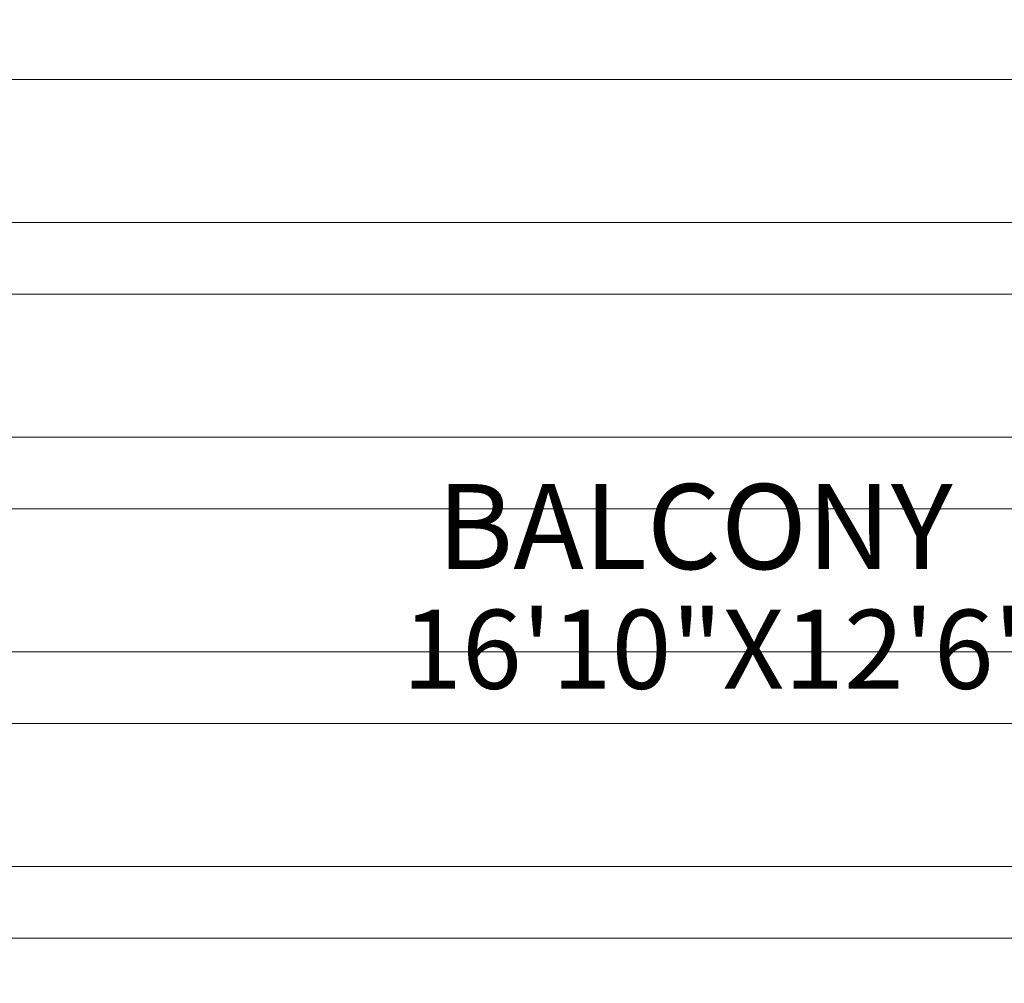
# Model space of a CAD drawing. Units: inches. Extents: x 351 to 1738, y -265 to 286.
# Tile 14 of 38: x 1090 to 1176, y -147 to -63. Entities that reach past the tile are written whole.
import ezdxf

# ---------------------------------------------------------------- set-up
doc = ezdxf.new("R2010")
doc.units = ezdxf.units.IN
doc.header["$MEASUREMENT"] = 0
doc.layers.add('A-AREA-IDEN', color=7, linetype='Continuous', lineweight=18)
doc.layers.add('A-FLOR-PATT', color=9, linetype='Continuous', lineweight=9)
doc.styles.add('Annotative', font='arial.ttf')

msp = doc.modelspace()

# ---------------------------------------------------------------- hatches: boundary and pattern name
at = {"layer": 'A-FLOR-PATT', "transparency": 33554559}
h = msp.add_hatch(dxfattribs=at)
h.set_pattern_fill('ANSI37', color=256, scale=200, angle=135)
h.set_pattern_definition([(180, (1112.704, -164.037), (-2e-15, -25), []), (270, (1112.704, -164.037), (25, -5e-15), [])])
h.paths.add_polyline_path([(1380.064, 73.463), (1380.132, 148.463), (1338.064, 148.463), (1290.704, 148.463), (1290.704, 88.463), (1248.704, 88.463), (1248.704, -2.009), (1244.704, -2.009), (1244.704, 142.457), (1160.704, 142.457), (1160.704, 158.963), (1160.704, 170.137), (1160.704, 206.137), (1160.704, 228.963), (1112.704, 228.963), (1112.704, 209.963), (1112.704, 168.963), (1124.704, 168.963), (1124.704, 162.963), (1112.704, 162.963), (1112.704, 64.463), (1112.704, 60.463), (1112.704, 0.463), (1112.704, -48.026), (1146.804, -47.981), (1146.804, -35.691), (1207.804, -35.691), (1207.804, -47.902), (1236.542, -47.864), (1236.544, -50.009), (1248.5, -50.009), (1248.506, -102.915), (1248.512, -150.915), (1248.514, -164.037), (1248.549, -164.037), (1273.017, -164.037), (1273.017, -128.799), (1355.24, -128.799), (1355.24, -164.037), (1384.204, -164.037), (1384.204, -57.037), (1380.064, -57.037), (1380.064, -48.037), (1392.064, -48.037), (1392.064, -53.037), (1406.549, -53.037), (1406.549, -57.037), (1401.204, -57.037), (1401.204, -147.037), (1468.204, -147.037), (1468.204, -138.5), (1472.204, -138.5), (1472.204, -102.5), (1468.204, -102.5), (1468.204, -57.037), (1442.549, -57.037), (1442.549, -53.037), (1463.049, -53.037), (1463.049, -40.747), (1524.049, -40.747), (1524.049, -48.037), (1536.064, -48.037), (1536.064, -53.037), (1557.704, -53.037), (1557.704, 204.963), (1384.204, 204.963), (1384.204, 73.463), (1392.064, 73.463), (1392.064, 64.463), (1384.204, 64.463), (1384.204, -3.5), (1380.204, -3.537), (1380.204, 64.463), (1380.064, 64.463)])
h.paths.add_polyline_path([(1510.714, 86.458, -0.103984), (1511.661, 85.595, 0.470438), (1510.158, 87.614, 0.0961)], flags=16)
h.paths.add_polyline_path([(1510.443, 100.266, 0.009798), (1504.693, 100.48, 0.02879), (1504.6, 99.767, -0.165331), (1505.519, 96.135, -0.143601)], flags=16)
h.paths.add_polyline_path([(1487.201, 85.595, -0.103984), (1488.148, 86.458, 0.0961), (1488.704, 87.614, 0.470438)], flags=0)
h.paths.add_polyline_path([(1495.052, 100.43), (1494.178, 100.43, -0.026463), (1494.262, 99.774, -0.144219)], flags=16)
h.paths.add_polyline_path([(1444.485, 86.458, -0.103984), (1445.433, 85.595, 0.470438), (1443.93, 87.614, 0.0961)], flags=16)
h.paths.add_polyline_path([(1420.972, 85.595, -0.103984), (1421.92, 86.458, 0.0961), (1422.475, 87.614, 0.470438)], flags=16)
h.paths.add_polyline_path([(1428.632, 100.335, 0.001054), (1427.971, 100.309, -0.021524), (1428.033, 99.774, -0.114301)], flags=16)
h.paths.add_polyline_path([(1419.906, 143.708, 0.024979), (1420.222, 157.526), (1421.573, 159.101), (1421.573, 175.369), (1391.393, 175.369), (1391.393, 200.519), (1542.294, 200.519), (1542.294, 175.369), (1512.028, 175.369, 0.019865), (1511.521, 153.838, 0.025134), (1512.758, 118.323, 0.020553), (1512.942, 115.253), (1419.834, 115.253, -0.000414), (1419.843, 124.798), (1413.059, 124.798), (1413.059, 84.437, -0.061853), (1415.831, 80.45, -0.093077), (1420.972, 85.595, -0.267537), (1422.371, 84.732, 0.08511), (1424.052, 84.616, -0.885393), (1424.033, 84.851, -1.125815), (1424.073, 84.366, -0.087987), (1422.371, 84.732, -0.267537), (1422.326, 83.089, -0.370542), (1420.972, 85.595, 0.093077), (1415.831, 80.45, -0.087414), (1417.914, 73.937), (1418.941, 73.937, 0.02725), (1418.913, 76.906, -0.115703), (1421.051, 73.937), (1445.354, 73.937, -0.115703), (1447.492, 76.906, 0.02725), (1447.464, 73.937), (1448.491, 73.937, -0.087414), (1450.574, 80.45, 0.093077), (1445.433, 85.595, -0.370542), (1444.079, 83.089, -0.267537), (1444.034, 84.732, -0.087987), (1442.332, 84.366, -1.125815), (1442.372, 84.851, -2.032736), (1442.364, 84.368, 0.086378), (1444.034, 84.732, -0.267537), (1445.433, 85.595, -0.093077), (1450.574, 80.45, -0.257732), (1466.483, 90.927, -0.47867), (1468.832, 91.907, -0.47867), (1471.18, 90.927, -0.26264), (1483.053, 81.78, -0.071866), (1487.201, 85.595, -0.267537), (1488.6, 84.732, 0.08511), (1490.28, 84.616, -0.885393), (1490.262, 84.851, -1.125815), (1490.301, 84.366, -0.087987), (1488.6, 84.732, -0.267537), (1488.554, 83.089, -0.370542), (1487.201, 85.595, 0.071866), (1483.053, 81.78, -0.132065), (1484.143, 73.937), (1485.169, 73.937, 0.02725), (1485.142, 76.906, -0.115703), (1487.28, 73.937), (1511.582, 73.937, -0.115703), (1513.72, 76.906, 0.02725), (1513.693, 73.937), (1514.719, 73.937, -0.087414), (1516.802, 80.45, 0.093077), (1511.661, 85.595, -0.370542), (1510.308, 83.089, -0.267537), (1510.262, 84.732, -0.087987), (1508.561, 84.366, -1.125815), (1508.601, 84.851, -2.032736), (1508.592, 84.368, 0.086378), (1510.262, 84.732, -0.267537), (1511.661, 85.595, -0.093077), (1516.802, 80.45, -0.061853), (1519.575, 84.437), (1519.575, 73.937), (1413.059, 73.937), (1413.059, 124.798), (1419.843, 124.798, -0.000821)], flags=16)
h.paths.add_polyline_path([(1220.149, 54.133, -0.103984), (1220.869, 53.476, 0.470438), (1219.727, 55.011, 0.0961)], flags=16)
h.paths.add_polyline_path([(1219.944, 64.626, 0.009798), (1215.574, 64.789, 0.02879), (1215.503, 64.247, -0.165331), (1216.201, 61.487, -0.143601)], flags=16)
h.paths.add_polyline_path([(1209.779, 64.449, 0.097446), (1209.339, 64.751), (1208.247, 64.751, 0.12739), (1207.7, 64.326, 0.171586), (1206.95, 61.475, -0.158854), (1207.636, 59.45, 0.015898), (1207.795, 59.218, 0.061546), (1208.598, 59.616, 0.175416), (1208.638, 60.099, -0.284779), (1209.348, 62.472, 0.326216)], flags=16)
h.paths.add_polyline_path([(1169.818, 54.133, -0.103984), (1170.538, 53.476, 0.470438), (1169.396, 55.011, 0.0961)], flags=16)
h.paths.add_polyline_path([(1159.017, 62.472, 0.284764), (1158.307, 60.099, -0.175433), (1158.267, 59.616, 0.39293), (1159.448, 64.449, -0.32623)], flags=16)
h.paths.add_polyline_path([(1156.342, 58.239, -0.178321), (1154.011, 55.31, -0.174736), (1154.722, 55.233, -0.200802), (1156.27, 56.086, 0.12699), (1157.283, 58.991, -0.091205)], flags=16)
h.paths.add_polyline_path([(1156.624, 61.413, 0.157275), (1157.316, 64.247, 0.169622)], flags=16)
h.paths.add_polyline_path([(1152.67, 54.133, -0.0961), (1151.95, 53.476, 0.064076), (1154.465, 54.384, 0.199016)], flags=16)
h.paths.add_polyline_path([(1202.281, 53.476, -0.103984), (1203, 54.133, 0.0961), (1203.423, 55.011, 0.470438)], flags=0)
h.paths.add_polyline_path([(1151.139, 97.64, 0.024979), (1151.379, 108.141), (1152.406, 109.338), (1152.406, 121.701), (1129.47, 121.701), (1129.47, 140.814), (1244.149, 140.814), (1244.149, 121.701), (1221.148, 121.701, 0.019865), (1220.763, 105.338, 0.025134), (1221.703, 78.349, 0.020553), (1221.843, 76.016), (1151.078, 76.016, -0.128743), (1148.786, 65.037, 0.539352), (1150.327, 64.171, -0.027594), (1163.481, 64.751, 0.097695), (1163.04, 64.449, 0.326216), (1163.471, 62.472, -0.284777), (1164.181, 60.099, -0.194757), (1165.846, 61.443, -0.155402), (1165.172, 64.247, -0.166022), (1165.869, 61.475, -0.177014), (1167.852, 62.77, -0.448203), (1169.974, 60.807, -0.393499), (1167.679, 57.86, -0.895548), (1168.438, 54.524, -0.355767), (1166.218, 56.086, -0.066024), (1165.505, 57.539), (1165.251, 56.243, -0.371732), (1164.02, 59.758, -0.373614), (1163.04, 64.449, -0.097695), (1163.481, 64.751, 0.021354), (1153.294, 64.429, -0.134183), (1156.695, 61.368, 0.186873), (1154.636, 62.77, 0.448203), (1152.514, 60.807, 0.403726), (1154.905, 57.846, 0.711219), (1153.334, 55, 0.53154), (1151.95, 53.476, -0.267537), (1153.013, 52.821, 0.08511), (1154.29, 52.732, -0.885393), (1154.276, 52.911, -1.125815), (1154.306, 52.543, -0.087987), (1153.013, 52.821, -0.267537), (1152.978, 51.572, -0.370542), (1151.95, 53.476, 0.093077), (1148.043, 49.566, -0.087414), (1149.626, 44.617), (1150.406, 44.617, 0.02725), (1150.385, 46.873, -0.115703), (1152.01, 44.617), (1170.478, 44.617, -0.115703), (1172.103, 46.873, 0.02725), (1172.082, 44.617), (1172.862, 44.617, -0.087414), (1174.445, 49.566, 0.093077), (1170.538, 53.476, -0.370542), (1169.51, 51.572, -0.267537), (1169.475, 52.821, -0.087987), (1168.182, 52.543, -1.125815), (1168.212, 52.911, -2.032736), (1168.206, 52.544, 0.086378), (1169.475, 52.821, -0.267537), (1170.538, 53.476, -0.093077), (1174.445, 49.566, -0.257732), (1186.536, 57.528, -0.47867), (1188.321, 58.273, -0.47867), (1190.106, 57.528, -0.26264), (1199.128, 50.577, -0.071866), (1202.281, 53.476, -0.267537), (1203.344, 52.821, 0.08511), (1204.621, 52.732, -0.885393), (1204.607, 52.911, -1.125815), (1204.637, 52.543, -0.087987), (1203.344, 52.821, -0.267537), (1203.309, 51.572, -0.370542), (1202.281, 53.476, 0.071866), (1199.128, 50.577, -0.132065), (1199.957, 44.617), (1200.737, 44.617, 0.02725), (1200.716, 46.873, -0.115703), (1202.341, 44.617), (1220.809, 44.617, -0.115703), (1222.434, 46.873, 0.02725), (1222.413, 44.617), (1223.193, 44.617, -0.087414), (1224.776, 49.566, 0.093077), (1220.869, 53.476, -0.370542), (1219.841, 51.572, -0.267537), (1219.806, 52.821, -0.087987), (1218.513, 52.543, -1.125815), (1218.543, 52.911, -2.032736), (1218.537, 52.544, 0.086378), (1219.806, 52.821, -0.267537), (1220.869, 53.476, -0.093077), (1224.776, 49.566, -0.061853), (1226.883, 52.597), (1226.883, 44.617), (1145.936, 44.617), (1145.936, 83.269), (1151.091, 83.269, -0.000821)], flags=16)
h.paths.add_polyline_path([(1218.01, 57.86, -0.895548), (1218.769, 54.524, -0.355767), (1216.549, 56.086, -0.066024), (1215.836, 57.539), (1215.582, 56.243, -0.371732), (1214.351, 59.758, -0.373614), (1213.371, 64.449, 0.326216), (1213.802, 62.472, -0.284777), (1214.512, 60.099, -0.194757), (1216.177, 61.443, -0.179991), (1218.183, 62.77, -0.448203), (1220.305, 60.807, -0.393499)], flags=16)
h.paths.add_polyline_path([(1424.735, 91.363, -0.393499), (1421.715, 95.241, -0.448203), (1424.507, 97.824, -0.179991), (1427.147, 96.077, -0.194757), (1429.338, 94.309, -0.284777), (1430.272, 97.432, 0.326216), (1430.839, 100.034, -0.373614), (1429.55, 93.861, -0.371732), (1427.929, 89.235), (1427.596, 90.941, -0.066024), (1426.657, 89.029, -0.355767), (1423.736, 86.973, -0.895548)], flags=16)
h.paths.add_polyline_path([(1238.033, 131.257, -1), (1227.329, 131.257, -1)], flags=0)
h.paths.add_polyline_path([(1235.357, 131.257, -1), (1230.005, 131.257, -1)], flags=0)
h.paths.add_polyline_path([(1214.039, 54.243, 0.154382), (1214.38, 53.992, 0.358955), (1213.613, 54.016, 0.603948), (1214.379, 53.657, 0.371319), (1213.968, 52.872, 0.187994), (1214.312, 52.809, -0.592455), (1213.953, 52.967, -0.294279), (1214.083, 53.691, -1.300187), (1213.881, 54.134, -0.283762), (1214.469, 53.896, 1.15094)], flags=16)
h.paths.add_polyline_path([(1212.091, 56.286, -0.408434), (1211.337, 56.445, -0.036259), (1211.098, 56.848, -0.236098), (1211.59, 56.63, 0.035345), (1211.835, 56.543, -0.475241), (1212.091, 56.286, -0.475241), (1212.438, 56.182, 0.035345), (1212.631, 56.007, -0.236098), (1213.056, 55.676, -0.036259), (1212.588, 55.697, -0.408434)], flags=16)
h.paths.add_polyline_path([(1211.469, 50.297, 0.296043), (1210.47, 50.527, 0.310883), (1211.931, 50.148, 0.021255)], flags=16)
h.paths.add_polyline_path([(1213.739, 51.818, -0.036259), (1213.271, 51.838, -0.408434), (1212.774, 52.427, -0.094786), (1212.293, 50.703, 1.150474), (1212.911, 50.232, 0.166288), (1213.265, 50.68, -0.025254), (1212.603, 50.13, 1.087932), (1212.471, 49.407, 0.166288), (1213.02, 49.251, -0.016128), (1212.567, 49.563, -0.286859), (1212.217, 49.638, 0.022156), (1212.046, 50.055, -0.64613), (1212.185, 50.498, 0.088412), (1212.732, 52.077, -1.186037), (1213.121, 52.323, 0.035345), (1213.314, 52.148, -0.236098)], flags=16)
h.paths.add_polyline_path([(1212.094, 50.342, -0.048524), (1211.54, 49.605, -1.103834), (1211.397, 48.738, -0.785515), (1211.683, 48.254, -0.392043), (1210.948, 48.525, -0.392819), (1210.561, 47.995, -0.592455), (1210.201, 48.153, -0.294279), (1210.331, 48.877, -0.704172), (1210.316, 49.592, -0.679344), (1210.729, 50.112, 0.563676)], flags=16)
h.paths.add_polyline_path([(1211.274, 49.829, -0.139826), (1210.745, 49.859, -0.217879), (1210.948, 49.509, -0.498572)], flags=0)
h.paths.add_polyline_path([(1433.426, 81.49, -0.181571), (1434.245, 81.788, -0.008067), (1433.726, 82.205, 0.045578), (1432.755, 81.242, 0.179011)], flags=16)
h.paths.add_polyline_path([(1434.146, 81.009, -0.132442), (1433.645, 80.771, 0.259089), (1433.234, 80.471, -0.180211), (1433.392, 80.805, -0.16994), (1432.758, 81.109, 0.032652), (1433.273, 80.474, -0.493363), (1434.046, 80.146, -0.390497)], flags=16)
h.paths.add_polyline_path([(1434.83, 80.047, -0.947538), (1435.294, 79.576, -0.299128), (1434.625, 79.404, -0.270439), (1435.01, 78.591, -0.592455), (1434.537, 78.382, -0.392819), (1434.027, 79.08, -0.392043), (1433.06, 78.723, -0.352042), (1433.003, 79.197, -0.197216), (1433.75, 79.734, -0.71364), (1434.447, 79.939, -0.21479), (1434.819, 80.475, 0.408833), (1435.075, 80.803, -0.226152)], flags=16)
h.paths.add_polyline_path([(1432.67, 81.217, -0.454218), (1431.897, 79.923, -0.414411), (1431.301, 80.035, 0.016129), (1431.897, 80.445, 0.27957), (1432.073, 80.871, -0.289504), (1431.103, 81.321, -0.414411), (1430.978, 81.915, 0.01613), (1431.586, 81.521, 0.341293), (1432.125, 81.583, -0.813186)], flags=16)
h.paths.add_polyline_path([(1429.893, 86.381, -0.947538), (1430.358, 85.91, -0.173106), (1429.984, 85.712, -0.038817), (1431.625, 84.214, -0.0879), (1432.097, 88.549, -0.049768), (1431.254, 88.49, -0.236098), (1431.814, 88.925, 0.035345), (1432.067, 89.155, -0.475241), (1432.524, 89.291, -0.475241), (1432.86, 89.63, 0.035345), (1433.182, 89.744, -0.236098), (1433.83, 90.032, -0.036259), (1433.516, 89.502, -0.408434), (1432.524, 89.291, -0.312424), (1432.106, 88.58, 0.088559), (1431.625, 84.214, -0.408434), (1430.971, 83.439, -0.036259), (1430.355, 83.412, -0.236098), (1430.914, 83.847, 0.035345), (1431.168, 84.078, -0.475241), (1431.625, 84.214, 0.038817), (1429.984, 85.712, -0.321732), (1429.333, 86.048, -0.32743), (1429.883, 86.809, 0.408833), (1430.138, 87.138, -0.226152)], flags=16)
h.paths.add_polyline_path([(1211.206, 58.616, -0.999784), (1211.336, 59.323, -0.614994)], flags=16)
h.paths.add_polyline_path([(1210.288, 49.429, 0.154382), (1210.629, 49.178, 0.358955), (1209.861, 49.202, 0.603948), (1210.627, 48.843, -0.534825), (1210.806, 49.295, 0.748346)], flags=16)
h.paths.add_polyline_path([(1209.589, 51.828, -0.008791), (1209.775, 51.753, 0.112231), (1209.466, 52.019, 1.418851), (1209.014, 51.708, -0.458726), (1208.651, 51.073, -0.592455), (1208.291, 51.232, -0.294279), (1208.421, 51.955, -1.300187), (1208.219, 52.398, -0.226005), (1208.719, 52.257, -0.475519), (1209.158, 52.369, -1.455499), (1209.603, 52.664, 0.421305), (1209.191, 52.262, -0.591212), (1208.979, 51.796, 0.497399), (1209.773, 51.333, 0.649312)], flags=16)
h.paths.add_polyline_path([(1208.029, 52.041, 0.544667), (1208.832, 52.045, 0.220132)], flags=0)
h.paths.add_polyline_path([(1210.438, 51.425, -0.2042), (1210.277, 52.018, 0.270826), (1209.915, 52.897, 0.324115)], flags=0)
h.paths.add_polyline_path([(1209.668, 52.407, -0.60139), (1208.99, 52.221, -0.394916), (1208.248, 52.83, -0.836792), (1208.651, 53.017, -0.338488), (1209.039, 52.571, 0.194138), (1209.191, 52.262, 0.413995), (1209.712, 52.475, 0.51771), (1210.503, 51.416, 0.401922), (1209.493, 50.93, 0.206396), (1209.516, 50.165, -0.319463), (1210.417, 51.418, -0.466635)], flags=16)
h.paths.add_polyline_path([(1206.601, 56.086, -0.355767), (1204.381, 54.524, -0.921198), (1205.236, 57.846, 0.206569), (1207.614, 58.991, -0.12699)], flags=16)
h.paths.add_polyline_path([(1435.487, 82.816, 0.527765), (1436.615, 83.361, 0.50854), (1437.05, 82.433, 0.592455), (1437.524, 82.641, 0.331245), (1436.963, 83.548, 0.387863), (1437.808, 83.626, 0.592954), (1437.618, 84.176, 0.226016), (1436.961, 83.99, 0.318205), (1437.588, 84.854, 0.689374), (1437.05, 84.991, 0.335765), (1436.539, 84.41, -0.156993), (1436.404, 84.065, -0.434611), (1436.961, 83.99, -0.21479), (1437.333, 84.526, 0.408833), (1437.588, 84.854, -0.226152), (1437.343, 84.097, -0.947538), (1437.808, 83.626, -0.299128), (1437.139, 83.455, -0.270439), (1437.524, 82.641, -0.592455), (1437.05, 82.433, -0.392819), (1436.541, 83.13, -0.43966), (1435.475, 82.794, -0.174614), (1435.942, 82.244, -0.206396), (1435.912, 81.237, -0.270826), (1435.125, 82.208, 0.207976), (1434.686, 82.904, -0.196495)], flags=16)
h.paths.add_polyline_path([(1435.386, 84.832, 0.270811), (1434.91, 83.676, -0.204217), (1434.699, 82.895, 0.324115)], flags=0)
h.paths.add_polyline_path([(1435.68, 84.18, -0.217656), (1435.554, 83.304, -0.176705), (1436.236, 83.778, -0.373036)], flags=0)
h.paths.add_polyline_path([(1435.566, 100.034, 0.326216), (1436.133, 97.432, -0.284777), (1437.067, 94.309, -0.194757), (1439.258, 96.077, -0.155402), (1438.371, 99.767, -0.166022), (1439.289, 96.12, -0.177014), (1441.897, 97.824, -0.448203), (1444.69, 95.241, -0.393499), (1441.67, 91.363, -0.895548), (1442.669, 86.973, -0.355767), (1439.748, 89.029, -0.066024), (1438.809, 90.941), (1438.476, 89.235, -0.371732), (1436.855, 93.861, -0.373614)], flags=16)
h.paths.add_polyline_path([(1191.252, 49.507, -0.274022), (1190.658, 48.409, 0.267537), (1191.311, 47.344, 0.370542)], flags=0)
h.paths.add_polyline_path([(1190.301, 49.717, 0.199016), (1188.619, 49.04, 0.064076), (1191.252, 49.507, -0.0961)], flags=0)
h.paths.add_polyline_path([(1189.518, 47.857, 1.125815), (1189.676, 47.523, 2.044605)], flags=0)
h.paths.add_polyline_path([(1464.974, 80.372, 0.274022), (1465.756, 78.927, -0.083013)], flags=0)
h.paths.add_polyline_path([(1464.974, 80.372, 0.370542), (1464.897, 77.525, 0.576324)], flags=0)
h.paths.add_polyline_path([(1464.974, 80.372, -0.470438), (1467.284, 81.372, -0.0961), (1466.226, 80.648, -0.199016), (1468.439, 79.757, -0.064076)], flags=0)
h.paths.add_polyline_path([(1189.511, 56.43, -0.259467), (1188.321, 56.391, -0.259467), (1187.13, 56.43, 0.08511), (1188.193, 55.716, -0.885393), (1188.27, 55.878, -1.196013), (1188.355, 55.442, 0.101459)], flags=0)
h.paths.add_polyline_path([(1188.321, 57.596, 0.078072), (1187.678, 57.24, 0.01555), (1188.321, 57.136, 0.01555), (1188.964, 57.24, 0.078072)], flags=0)
h.paths.add_polyline_path([(1190.164, 55.365, -0.576324), (1190.106, 57.528, -0.198294), (1188.321, 58.319, -0.198294), (1186.536, 57.528, -0.576324), (1186.477, 55.365, -0.370542), (1186.536, 57.528, 0.198294), (1188.321, 58.319, 0.198294), (1190.106, 57.528, -0.370542)], flags=0)
h.paths.add_polyline_path([(1188.372, 55.878, 1.125814), (1188.529, 55.544, 2.044605)], flags=0)
h.paths.add_polyline_path([(1186.341, 49.717, -0.0961), (1185.389, 49.507, 0.064076), (1188.022, 49.04, 0.199016)], flags=0)
h.paths.add_polyline_path([(1185.389, 49.507, -0.267537), (1185.984, 48.409, 0.08511), (1187.046, 47.695, -0.885393), (1187.123, 47.857, -1.125815), (1186.966, 47.523, -0.087987), (1185.984, 48.409, -0.267537), (1185.331, 47.344, -0.370542)], flags=0)
h.paths.add_polyline_path([(1399.441, 187.944, -1), (1413.525, 187.944, -1)], flags=0)
h.paths.add_polyline_path([(1402.962, 187.944, -1), (1410.004, 187.944, -1)], flags=0)
h.paths.add_polyline_path([(1357.663, -72.245), (1377.272, -72.245), (1377.272, -91.854), (1357.663, -91.854)], flags=16)
h.paths.add_polyline_path([(1467.256, 78.201, -1.125815), (1467.049, 77.761, -2.044605)], flags=0)
h.paths.add_polyline_path([(1468.822, 88.714, 0.941125), (1469.106, 88.316, 1.137152), (1468.765, 88.755, 0.890986), (1468.99, 88.245, 0.094828), (1470.398, 89.481, -0.267537), (1471.18, 90.927, -0.028123), (1469.678, 90.547, -0.028774), (1469.948, 90.311, -0.020327), (1468.832, 90.41, -0.020327), (1467.716, 90.311, -0.028774), (1467.986, 90.547, -0.028123), (1466.483, 90.927, -0.267537), (1467.265, 89.481, 0.08511), (1468.663, 88.542, -1.202316)], flags=0)
h.paths.add_polyline_path([(1178.25, 124.523, -0.119929), (1165.65, 124.145, -0.107349), (1159.133, 124.446, -0.102891), (1159.132, 130.465, -0.074897), (1158.993, 137.956, 0.002027), (1167.844, 137.479, -0.07553), (1180.337, 137.666, -0.075861), (1186.502, 137.688, -0.14099), (1186.272, 130.046, -0.095481), (1186.729, 124.748, -0.10603)], flags=0)
h.paths.add_polyline_path([(1469.225, 79.757, -0.199016), (1471.437, 80.648, -0.0961), (1470.379, 81.372, -0.470438), (1472.689, 80.372, -0.370542), (1472.766, 77.525, -0.267537), (1471.907, 78.927, -0.087986), (1470.615, 77.761, -1.125849), (1470.408, 78.201, -2.032736), (1470.642, 77.778, 0.086378), (1471.907, 78.927, -0.267537), (1472.689, 80.372, -0.064076)], flags=0)
h.paths.add_polyline_path([(1430.423, 186.902, -0.074897), (1430.24, 196.758, 0.002027), (1441.887, 196.131, -0.07553), (1458.326, 196.377, -0.075861), (1466.438, 196.406, -0.14099), (1466.136, 186.35, -0.095481), (1466.737, 179.378, -0.10603), (1455.58, 179.082, -0.119929), (1439, 178.585, -0.107349), (1430.425, 178.981, -0.102891)], flags=0)
h.paths.add_polyline_path([(1162.258, 49.939, 0.335765), (1161.87, 49.497, -0.156994), (1161.767, 49.235, -0.434611), (1162.19, 49.178, -0.21479), (1162.473, 49.585, 1.529195)], flags=16)
h.paths.add_polyline_path([(1161.683, 49.021, 0.581518), (1161.268, 49.583, 0.592761)], flags=16)
h.paths.add_polyline_path([(1162.602, 48.058, 0.371319), (1162.192, 48.843, 0.434533), (1162.88, 48.962, 0.185081), (1162.197, 48.926, 1.121837)], flags=16)
h.paths.add_polyline_path([(1161.443, 48.941, -1.307104), (1161.495, 48.571, -0.217752), (1161.136, 48.254, 0.697303), (1161.871, 49.048, 0.121514)], flags=16)
h.paths.add_polyline_path([(1162.531, 49.429, -0.207084), (1162.05, 49.146, -0.99203)], flags=16)
h.paths.add_polyline_path([(1161.304, 49.578, -0.719667), (1161.513, 50.079, -0.130428), (1160.836, 50.168, 0.039593)], flags=0)
h.paths.add_polyline_path([(1162.036, 50.584, -0.008067), (1161.642, 50.9, 0.029367), (1161.35, 50.297, -0.205788)], flags=16)
h.paths.add_polyline_path([(1162.882, 51.392, -0.124733), (1162.763, 51.828, -0.101191), (1162.399, 51.438, -0.153425)], flags=0)
h.paths.add_polyline_path([(1164.235, 51.85, -0.309107), (1164.513, 51.136, -0.627125), (1163.781, 51.603, -0.685909), (1162.777, 51.219, -0.233285), (1163.303, 50.165, -0.270826), (1162.705, 50.903, 0.2042), (1162.381, 51.425, 0.204182), (1162.542, 52.018, -0.270841), (1162.903, 52.897, -0.127261), (1163.219, 52.529, -1.168681), (1163.781, 52.587, -0.329112), (1164.168, 53.017, -0.836792), (1164.571, 52.83, -0.193341), (1164.391, 52.338, -0.947538), (1164.744, 51.981, -0.299128)], flags=16)
h.paths.add_polyline_path([(1163.598, 51.937, -1.262956), (1163.236, 51.831, 0.012575), (1162.971, 51.721, 0.230657), (1163.151, 52.407, -0.164898), (1163.178, 52.661, -0.44932), (1163.628, 52.262, -0.721477), (1164.154, 52.088, -0.849998)], flags=0)
h.paths.add_polyline_path([(1161.613, 58.616, -0.980413), (1161.525, 59.049, -2.908935)], flags=16)
h.paths.add_polyline_path([(1160.252, 49.166, -0.414411), (1159.799, 49.251, 0.016129), (1160.252, 49.563, 0.27957), (1160.386, 49.887, -0.289504), (1159.649, 50.229, -0.414411), (1159.554, 50.68, 0.01613), (1160.015, 50.381, 0.617885), (1160.526, 50.703, -0.094786), (1160.045, 52.427, -0.140444), (1159.682, 52.042, -0.057856), (1159.3, 51.872, 0.544843), (1160.046, 52.419, -0.088122), (1160.404, 55.721, -0.049768), (1159.763, 55.676, -0.236098), (1160.188, 56.007, 0.035345), (1160.381, 56.182, -0.475241), (1160.728, 56.286, -0.475241), (1160.984, 56.543, 0.035345), (1161.229, 56.63, -0.236098), (1161.721, 56.848, -0.036259), (1161.482, 56.445, -0.408434), (1160.728, 56.286, -0.312424), (1160.411, 55.745, 0.088559), (1160.045, 52.427, 0.107081), (1160.634, 50.498, -0.494798), (1160.839, 50.149, -0.454218)], flags=16)
h.paths.add_polyline_path([(1160.666, 49.808, -2.076528), (1160.828, 50.172, 0.019586)], flags=0)
h.paths.add_polyline_path([(1158.439, 53.992, 0.154382), (1158.78, 54.243, 0.748346), (1158.262, 54.109, -0.338225), (1158.492, 53.839, -0.170816), (1159.124, 53.779, 0.495729), (1158.938, 54.134, 0.226016)], flags=16)
h.paths.add_polyline_path([(1160.045, 52.427, 0.038817), (1158.798, 53.565, -0.119818), (1158.574, 53.586, -0.309107), (1158.851, 52.872, -0.187994), (1158.506, 52.809, 0.592455), (1158.866, 52.967, 0.331245), (1158.44, 53.657, 0.201245), (1158.798, 53.565, -0.034023), (1159.901, 52.578, -0.044253), (1159.698, 52.323, -0.475241)], flags=16)
h.paths.add_polyline_path([(1336.926, -95.392), (1336.926, -117.945), (1291.82, -117.945), (1291.82, -95.392)], flags=16)
h.paths.add_polyline_path([(1357.535, -97.244), (1357.726, -96.697, 0.034844)], flags=16)
h.paths.add_polyline_path([(1376.693, -96.478), (1377.301, -96.5, 0.031497), (1375.907, -96.424), (1357.726, -96.424)], flags=16)
h.paths.add_polyline_path([(1379.403, -119.667, 0.026706), (1380.043, -119.439, -0.015299)], flags=16)
h.paths.add_polyline_path([(1357.726, -120.202), (1357.821, -120.202), (1357.821, -120.201)], flags=16)
h.paths.add_polyline_path([(1354.171, -104.592), (1354.469, -98.672, 0.011138)], flags=16)
h.paths.add_polyline_path([(1355.058, -119.136), (1354.578, -118.539, 0.143164)], flags=16)
h.paths.add_polyline_path([(1378.851, -96.821), (1378.85, -96.82), (1378.85, -96.82, -0.04968), (1380.055, -97.191), (1378.85, -96.82, 0.150054), (1375.135, -97.188), (1375.136, -119.44, -0.00997), (1374.747, -116.649), (1357.726, -116.649, 0.169385), (1357.535, -119.382), (1357.535, -119.382), (1357.535, -119.382, 0.034818), (1357.726, -119.928), (1357.726, -119.928), (1357.726, -119.929, -0.034877), (1357.535, -119.382), (1355.507, -119.382), (1355.317, -119.278), (1357.535, -119.382, -0.169394), (1357.726, -116.649, -0.039151), (1374.686, -116.113, -0.002015), (1374.625, -115.546, 0.115322), (1369.915, -115.474, 0.060921), (1369.922, -101.154, 0.115146), (1374.625, -101.079, -0.002016), (1374.686, -100.513, -0.039151), (1357.726, -99.977), (1374.747, -99.977, -0.009963), (1375.135, -97.188), (1375.135, -97.188, -0.150108)], flags=16)
h.paths.add_polyline_path([(1490.963, 91.363, -0.393499), (1487.944, 95.241, -0.448203), (1490.736, 97.824, -0.179991), (1493.376, 96.077, -0.194757), (1495.567, 94.309, -0.284777), (1496.501, 97.432, 0.326216), (1497.068, 100.034, -0.373614), (1495.778, 93.861, -0.371732), (1494.158, 89.235), (1493.824, 90.941, -0.066024), (1492.886, 89.029, -0.355767), (1489.964, 86.973, -0.895548)], flags=16)
h.paths.add_polyline_path([(1354.86, -97.658), (1355.316, -97.348, 0.101911)], flags=16)
h.paths.add_polyline_path([(1497.063, 83.327, 0.176724), (1496.37, 83.785, -0.405139), (1496.016, 83.384, 0.497399), (1497.06, 82.774, 0.649312), (1496.818, 83.426, -0.008791)], flags=16)
h.paths.add_polyline_path([(1496.339, 83.783, 0.592761), (1496.886, 84.522, 0.581518)], flags=16)
h.paths.add_polyline_path([(1495.11, 82.641, 0.592455), (1495.583, 82.433, 0.676915), (1495.805, 83.59, 0.375669)], flags=16)
h.paths.add_polyline_path([(1495.015, 84.176, -0.145057), (1495.301, 84.526, -0.408833), (1495.045, 84.854, 0.220629), (1495.381, 84.152, -0.199594), (1495.851, 83.764, -0.524017), (1494.826, 83.626, -0.592998)], flags=16)
h.paths.add_polyline_path([(1501.655, 81.915, -0.016129), (1501.048, 81.521, -0.392719), (1500.462, 81.37, -0.21067), (1500.607, 81.142, 0.306699)], flags=16)
h.paths.add_polyline_path([(1500.11, 89.291, -0.408434), (1499.118, 89.502, -0.036259), (1498.803, 90.032, -0.236098), (1499.451, 89.744, 0.035345), (1499.774, 89.63, -0.475241), (1500.11, 89.291, -0.475241), (1500.567, 89.155, 0.035345), (1500.82, 88.925, -0.236098), (1501.379, 88.49, -0.036259), (1500.763, 88.516, -0.408434)], flags=16)
h.paths.add_polyline_path([(1498.908, 82.205, -0.051322), (1500.013, 81.134, -0.587931), (1500.234, 81.676, 0.107081), (1501.009, 84.214, -0.03529)], flags=16)
h.paths.add_polyline_path([(1496.93, 83.875, -0.206396), (1497.247, 84.832, -0.270826), (1497.724, 83.676, 0.207976), (1497.944, 82.884, -0.381455)], flags=16)
h.paths.add_polyline_path([(1496.721, 81.237, 0.270812), (1497.509, 82.208, -0.204216), (1497.935, 82.895, 0.324115)], flags=16)
h.paths.add_polyline_path([(1497.529, 80.125, -0.145057), (1497.814, 80.475, -0.703182), (1498.282, 81.178, -0.122925), (1497.977, 81.714, -0.270837), (1499.207, 81.49, 0.207964), (1499.993, 81.248, -0.265145), (1499.278, 80.472, 0.381901), (1498.808, 79.947, -0.305905), (1498.848, 79.519, 0.499482), (1498.574, 79.217, -0.458726), (1498.097, 78.382, -0.592455), (1497.624, 78.591, -0.270439), (1498.009, 79.404, -0.299116), (1497.34, 79.576, -0.593016)], flags=16)
h.paths.add_polyline_path([(1500.736, 79.923, 0.414411), (1501.333, 80.035, -0.321648), (1500.192, 80.765, 0.019886), (1499.976, 81.251, 0.465331)], flags=16)
h.paths.add_polyline_path([(1501.009, 84.214, -0.038817), (1502.649, 85.712, -0.173095), (1502.276, 85.91, -0.593016), (1502.465, 86.46, -0.145057), (1502.751, 86.809, -0.408833), (1502.495, 87.138, 0.220629), (1502.831, 86.436, -0.199594), (1503.301, 86.048, -0.321732), (1502.649, 85.712, 0.038817), (1501.009, 84.214, 0.122449), (1501.412, 83.755, 0.475491), (1501.335, 84.226, 0.055822), (1501.719, 83.847, -0.236098), (1502.278, 83.412, -0.036259), (1501.663, 83.439, -0.408434)], flags=16)
h.paths.add_polyline_path([(1501.794, 100.034, 0.326216), (1502.362, 97.432, -0.284777), (1503.295, 94.309, -0.194757), (1505.486, 96.077, -0.179991), (1508.126, 97.824, -0.448203), (1510.918, 95.241, -0.393499), (1507.899, 91.363, -0.895548), (1508.898, 86.973, -0.355767), (1505.976, 89.029, -0.066024), (1505.038, 90.941), (1504.704, 89.235, -0.371732), (1503.084, 93.861, -0.373614)], flags=16)
h.paths.add_polyline_path([(1146.29, 131.257, -1), (1135.587, 131.257, -1)], flags=0)
h.paths.add_polyline_path([(1143.614, 131.257, -1), (1138.262, 131.257, -1)], flags=0)
h.paths.add_polyline_path([(1524.064, 73.463), (1536.064, 73.463), (1536.064, 64.463), (1524.064, 64.463)], flags=16)
h.paths.add_polyline_path([(1520.162, 187.944, -1), (1534.246, 187.944, -1)], flags=0)
h.paths.add_polyline_path([(1530.725, 187.944), (1527.204, 187.944), (1527.204, 184.423, 0.414214)], flags=0)
h.paths.add_polyline_path([(1278.415, -91.154), (1331.067, -91.154), (1331.067, -80.583), (1278.415, -80.583)], flags=24)
h.paths.add_polyline_path([(1266.655, -79.354), (1354.738, -79.354), (1354.738, -67.817), (1266.655, -67.817)], flags=24)
h.paths.add_polyline_path([(1115.482, 206.184), (1155.098, 206.184), (1155.098, 217.714), (1115.482, 217.714)], flags=24)
h.paths.add_polyline_path([(1161.771, 8.501), (1222.466, 8.501), (1222.466, 19.079), (1161.771, 19.079)], flags=24)
h.paths.add_polyline_path([(1164.656, 18.795), (1210.615, 18.795), (1210.615, 30.324), (1164.656, 30.324)], flags=24)
h.paths.add_polyline_path([(1368.147, -32.882), (1379.362, -32.882), (1379.362, -21.733), (1368.147, -21.733)], flags=24)
h.paths.add_polyline_path([(1244.842, -31.012), (1256.057, -31.012), (1256.057, -19.863), (1244.842, -19.863)], flags=24)
h.paths.add_polyline_path([(1114.589, 195.739), (1156.517, 195.739), (1156.517, 206.31), (1114.589, 206.31)], flags=24)
h.paths.add_polyline_path([(1436.398, 37.632), (1505.131, 37.632), (1505.131, 48.203), (1436.398, 48.203)], flags=24)
h.paths.add_polyline_path([(1435.991, 47.919), (1507.906, 47.919), (1507.906, 59.456), (1435.991, 59.456)], flags=24)
h.paths.add_polyline_path([(1415.107, -124.896), (1457.038, -124.896), (1457.038, -114.318), (1415.107, -114.318)], flags=24)
h.paths.add_polyline_path([(1417.992, -114.602), (1457.609, -114.602), (1457.609, -103.073), (1417.992, -103.073)], flags=24)
h = msp.add_hatch(dxfattribs=at)
h.set_pattern_fill('ANSI32', color=256, scale=50, angle=135)
h.set_pattern_definition([(180, (1038.704, -199.037), (-2e-15, -18.75), []), (180, (1032.454, -192.787), (-2e-15, -18.75), [])])
h.paths.add_polyline_path([(1248.506, -102.915), (1236.559, -102.916), (1236.553, -56.864), (1112.704, -57.026), (1112.704, -57.037), (1103.704, -57.037), (1103.704, -45.037), (1103.704, 98.963), (1076.434, 98.963), (1076.549, -81.037), (1071.549, -81.037), (1043.704, -81.037), (1038.704, -81.037), (1038.704, -161.037), (1043.704, -161.037), (1043.704, -173.037), (1038.704, -173.037), (1038.704, -199.037), (1562.704, -199.037), (1562.704, -173.037), (1236.549, -173.037), (1236.549, -164.037), (1236.693, -164.037), (1236.676, -150.916), (1248.512, -150.915)])
h.paths.add_polyline_path([(1236.133, -134.078), (1247.348, -134.078), (1247.348, -122.929), (1236.133, -122.929)], flags=24)
h.paths.add_polyline_path([(1308.144, -185.548), (1321.66, -185.548), (1321.66, -174.4), (1308.144, -174.4)], flags=24)
h.paths.add_polyline_path([(1121.632, -122.88), (1179.647, -122.88), (1179.647, -112.309), (1121.632, -112.309)], flags=24)
h.paths.add_polyline_path([(1124.515, -112.593), (1177.986, -112.593), (1177.986, -101.056), (1124.515, -101.056)], flags=24)
h.paths.add_polyline_path([(1091.374, 23.58), (1104.89, 23.58), (1104.89, 34.728), (1091.374, 34.728)], flags=24)

# ---------------------------------------------------------------- texts
at = {"layer": 'A-AREA-IDEN', "style": 'Annotative'}
for s, height, p in [('BALCONY', 7.4326, (1126.438, -110.543)), ('16\'10"X12\'6"', 6.90137, (1123.394, -121))]:
    msp.add_text(s, height=height, dxfattribs=at).set_placement(p)

doc.saveas('drawing.dxf')
